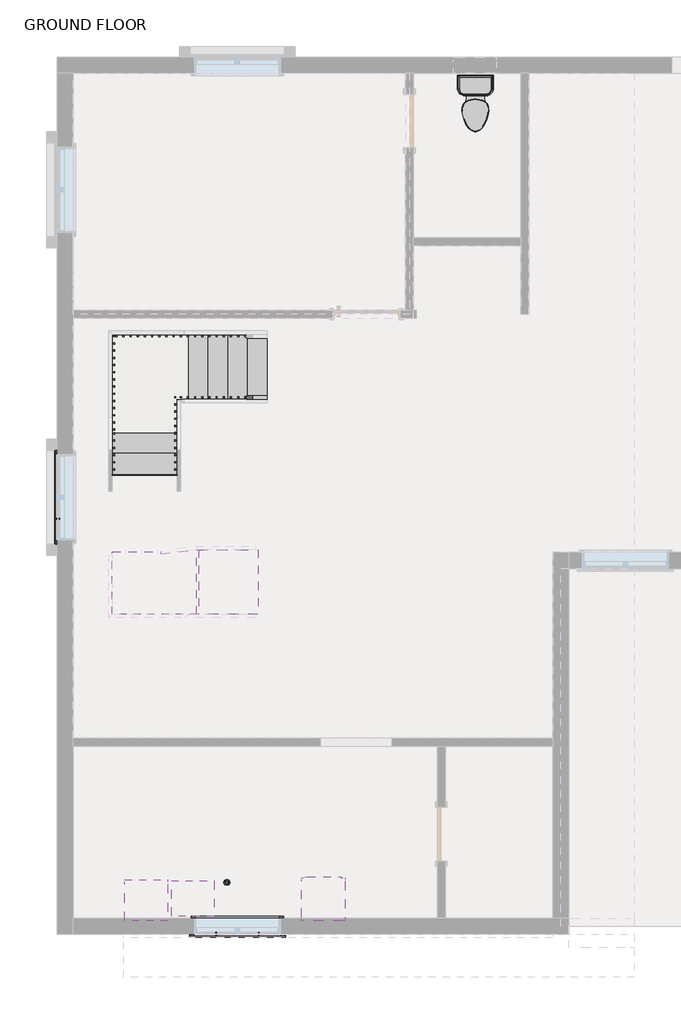
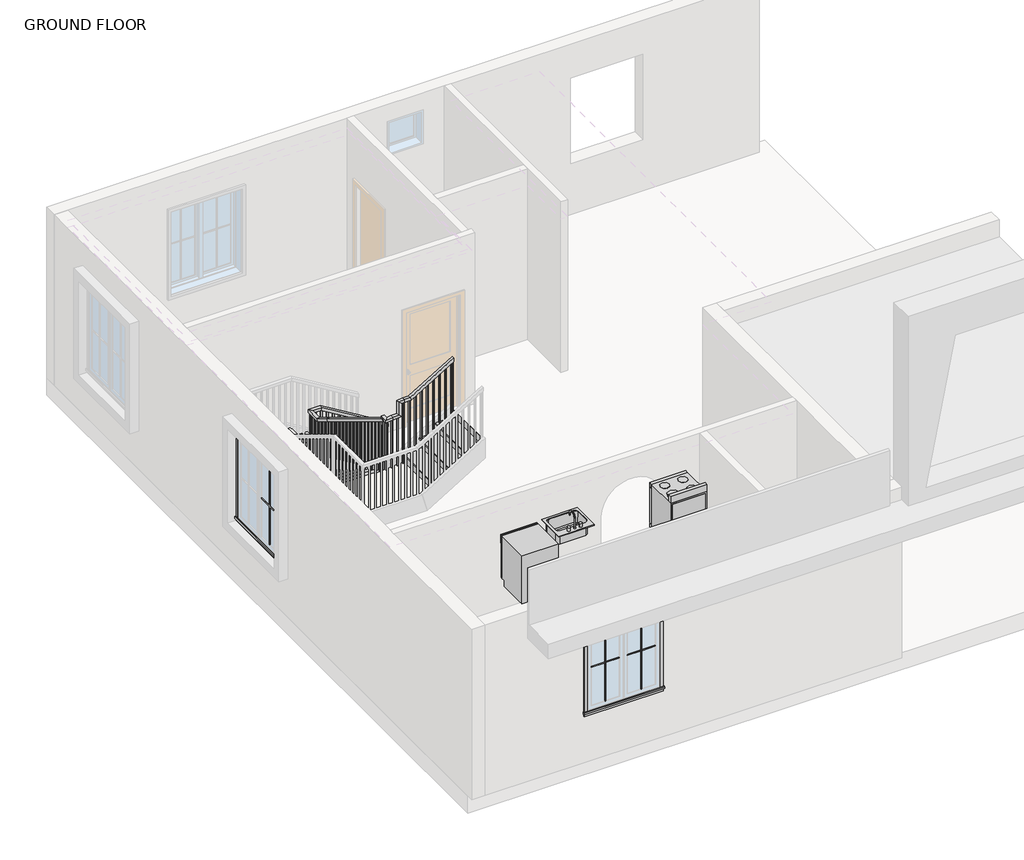
# One storey, part 3 of 4: 8 proxies, 3 flow terminals, 3 stair flights, 2 slabs, 1 railing.
"""IFC4 building model written with IfcOpenShell, lengths in millimetres."""

from ifc_helpers import new_model, si_unit, frame, origin, place, context, project, spatial, polyline, outline, extrude, faceted_brep, transform, mapped, element, save
from components import dishwasher_m_610_x_610_x_860mm_59039f12, muntin_pattern_2x2_muntin_pattern_2x2_6dad3731, muntin_pattern_2x2_muntin_pattern_2x2_a30a3345, range_m_610_x_610mm_7142e668, trim_window_exterior_flat_with_sill_92b9b949, trim_window_interior_flat_picture_frame_3bb882cf, flow_terminal_64mm_drain_64mm_drain_371441a0, m_sink_kitchen_single_760_x_535mm_2_7dd6f654, toilet_domestic_3d_toilet_domestic_3d_ba6479b0, toilet_domestic_3d_toilet_domestic_3d_30431060, non_monolithic_landing_bb2b3a88, non_monolithic_landing_7f41dad4, stair_flight_b4bfd778, stair_flight_23f0772b, stair_flight_a2e4d9b1

model = new_model("IFC4")

# Units and contexts
model_context = context("Model", 3, world=origin())
ifc_project = project(units=[si_unit("LENGTHUNIT", "METRE", prefix="MILLI")], contexts=[model_context])

# Site, building, storey
site = spatial("IfcSite", under=ifc_project)
building = spatial("IfcBuilding", under=site)
storey = spatial("IfcBuildingStorey", under=building, Name="GROUND FLOOR", Elevation=304.8)

# Proxies
placement = place(None, origin())
dishwasher_m_610_x_610_x_860mm_shape = dishwasher_m_610_x_610_x_860mm_59039f12(model_context)
element("IfcBuildingElementProxy", 1, Name="Dishwasher (M) : 610 x 610 x 860mm", ObjectType="Dishwasher (M) : 610 x 610 x 860mm", at=placement, inside=storey, context=model_context, shape_type="MappedRepresentation", body=[
    mapped(dishwasher_m_610_x_610_x_860mm_shape, transform((-11169.8760692, -6687.8348469, 3352.8), x_axis=(1.0, 0.0, 0.0), y_axis=(0.0, 1.0, 0.0), z_axis=(0.0, 0.0, 1.0))),
])
muntin_pattern_2x2_muntin_pattern_2x2_shape = muntin_pattern_2x2_muntin_pattern_2x2_6dad3731(model_context)
element("IfcBuildingElementProxy", 2, Name="Muntin Pattern_2x2 : Muntin Pattern_2x2", ObjectType="Muntin Pattern_2x2 : Muntin Pattern_2x2", at=placement, inside=storey, context=model_context, shape_type="MappedRepresentation", body=[
    mapped(muntin_pattern_2x2_muntin_pattern_2x2_shape, transform((-9193.7461008, -7440.4594117, 1289.05), x_axis=(-1.0, 0.0, 0.0), y_axis=(0.0, -1.0, 0.0), z_axis=(0.0, 0.0, 1.0))),
])
element("IfcBuildingElementProxy", 3, Name="Muntin Pattern_2x2 : Muntin Pattern_2x2", ObjectType="Muntin Pattern_2x2 : Muntin Pattern_2x2", at=placement, inside=storey, context=model_context, shape_type="MappedRepresentation", body=[
    mapped(muntin_pattern_2x2_muntin_pattern_2x2_shape, transform((-12040.1336008, -1561.9469117, 1289.05), x_axis=(0.0, 1.0, 0.0), y_axis=(-1.0, 0.0, 0.0), z_axis=(0.0, 0.0, 1.0))),
])
muntin_pattern_2x2_muntin_pattern_2x2_2_shape = muntin_pattern_2x2_muntin_pattern_2x2_a30a3345(model_context)
element("IfcBuildingElementProxy", 4, Name="Muntin Pattern_2x2 : Muntin Pattern_2x2", ObjectType="Muntin Pattern_2x2 : Muntin Pattern_2x2", at=placement, inside=storey, context=model_context, shape_type="MappedRepresentation", body=[
    mapped(muntin_pattern_2x2_muntin_pattern_2x2_2_shape, transform((-9800.1711008, -7440.4594117, 1289.05), x_axis=(1.0, 0.0, 0.0), y_axis=(0.0, 1.0, 0.0), z_axis=(0.0, 0.0, 1.0))),
])
range_m_610_x_610mm_shape = range_m_610_x_610mm_7142e668(model_context)
element("IfcBuildingElementProxy", 5, Name="Range (M) : 610 x 610mm", ObjectType="Range (M) : 610 x 610mm", at=placement, inside=storey, context=model_context, shape_type="MappedRepresentation", body=[
    mapped(range_m_610_x_610mm_shape, transform((-8584.7586008, -6649.4844117, 3352.8), x_axis=(1.0, 0.0, 0.0), y_axis=(0.0, 1.0, 0.0), z_axis=(0.0, 0.0, 1.0))),
])
trim_window_exterior_flat_with_sill_shape = trim_window_exterior_flat_with_sill_92b9b949(model_context)
element("IfcBuildingElementProxy", 6, Name="Trim-Window-Exterior-Flat : with Sill", ObjectType="Trim-Window-Exterior-Flat : with Sill", at=placement, inside=storey, context=model_context, shape_type="MappedRepresentation", body=[
    mapped(trim_window_exterior_flat_with_sill_shape, transform((-9496.9586008, -7449.9844117, 2743.2), x_axis=(1.0, 0.0, 0.0), y_axis=(0.0, 0.0, 1.0), z_axis=(0.0, -1.0, 0.0))),
])
element("IfcBuildingElementProxy", 7, Name="Trim-Window-Exterior-Flat : with Sill", ObjectType="Trim-Window-Exterior-Flat : with Sill", at=placement, inside=storey, context=model_context, shape_type="MappedRepresentation", body=[
    mapped(trim_window_exterior_flat_with_sill_shape, transform((-12049.6586008, -1258.7344117, 2743.2), x_axis=(0.0, -1.0, 0.0), y_axis=(0.0, 0.0, 1.0), z_axis=(-1.0, 0.0, 0.0))),
])
trim_window_interior_flat_picture_frame_shape = trim_window_interior_flat_picture_frame_3bb882cf(model_context)
element("IfcBuildingElementProxy", 8, Name="Trim-Window-Interior-Flat : Picture Frame", ObjectType="Trim-Window-Interior-Flat : Picture Frame", at=placement, inside=storey, context=model_context, shape_type="MappedRepresentation", body=[
    mapped(trim_window_interior_flat_picture_frame_shape, transform((-9496.9586008, -7221.3844117, 2743.2), x_axis=(-1.0, 0.0, 0.0), y_axis=(0.0, 0.0, 1.0), z_axis=(0.0, 1.0, 0.0))),
])

# Flow terminals
flow_terminal_64mm_drain_64mm_drain_shape = flow_terminal_64mm_drain_64mm_drain_371441a0(model_context)
element("IfcFlowTerminal", 9, ObjectType="64mm Drain : 64mm Drain", at=placement, inside=storey, context=model_context, shape_type="MappedRepresentation", body=[
    mapped(flow_terminal_64mm_drain_64mm_drain_shape, transform((-9497.2638536, -6711.8269352, 1092.2555314), x_axis=(1.0, 0.0, 0.0), y_axis=(0.0, 1.0, 0.0), z_axis=(0.0, 0.0, 1.0))),
])
m_sink_kitchen_single_760_x_535mm_2_shape = m_sink_kitchen_single_760_x_535mm_2_7dd6f654(model_context)
element("IfcFlowTerminal", 10, ObjectType="M_Sink Kitchen-Single : 760 x 535mm 2", at=placement, inside=storey, context=model_context, shape_type="MappedRepresentation", body=[
    mapped(m_sink_kitchen_single_760_x_535mm_2_shape, transform((-10114.0693602, -6939.4390106, 3352.8), x_axis=(-1.0, 0.0, 0.0), y_axis=(0.0, -1.0, 0.0), z_axis=(0.0, 0.0, 1.0))),
])
toilet_domestic_3d_toilet_domestic_3d_shape = toilet_domestic_3d_toilet_domestic_3d_ba6479b0(model_context)
toilet_domestic_3d_toilet_domestic_3d_2_shape = toilet_domestic_3d_toilet_domestic_3d_30431060(model_context)
element("IfcFlowTerminal", 11, ObjectType="Toilet-Domestic-3D : Toilet-Domestic-3D", at=placement, inside=storey, context=model_context, shape_type="MappedRepresentation", body=[
    mapped(toilet_domestic_3d_toilet_domestic_3d_shape, transform((-6125.1086008, 4221.3155883, 304.8), x_axis=(1.0, 0.0, 0.0), y_axis=(0.0, 1.0, 0.0), z_axis=(0.0, 0.0, 1.0))),
    mapped(toilet_domestic_3d_toilet_domestic_3d_2_shape, transform((-6125.1086008, 4221.3155883, 304.8), x_axis=(1.0, 0.0, 0.0), y_axis=(0.0, 1.0, 0.0), z_axis=(0.0, 0.0, 1.0))),
])

# Railing
element("IfcRailing", 12, ObjectType="Handrail - Rectangular", at=placement, inside=storey, context=model_context, shape_type="SolidModel", body=[
    faceted_brep([(-9079.7156858, 130.7115003, 1388.5333333), (-9079.7156858, 130.7115003, 1329.1318731), (-9079.7156858, 181.5115003, 1329.1318731), (-9079.7156858, 181.5115003, 1388.5333333), (-10197.3156858, 130.7115003, 2065.8666667), (-10211.5080953, 130.7115003, 2015.0666667), (-10211.5080953, 181.5115003, 2015.0666667), (-10197.3156858, 181.5115003, 2065.8666667), (-10353.7522729, 130.7115003, 2065.8666667), (-10353.7522729, 130.7115003, 2015.0666667), (-10404.5522729, 181.5115003, 2015.0666667), (-10404.5522729, 181.5115003, 2065.8666667), (-10353.7522729, -76.9993654, 2065.8666667), (-10353.7522729, -91.1917748, 2015.0666667), (-10404.5522729, -91.1917748, 2015.0666667), (-10404.5522729, -76.9993654, 2065.8666667), (-10353.7522729, -356.3993654, 2235.2), (-10353.7522729, -382.7290926, 2191.7559502), (-10404.5522729, -382.7290926, 2191.7559502), (-10404.5522729, -356.3993654, 2235.2), (-10353.7522729, -1959.5850154, 3206.8276667), (-10353.7522729, -2010.3850154, 3178.2140852), (-10404.5522729, -2010.3850154, 3178.2140852), (-10404.5522729, -1959.5850154, 3206.8276667), (-10353.7522729, -1959.5850154, 3251.2), (-10353.7522729, -2010.3850154, 3200.4), (-10404.5522729, -2010.3850154, 3200.4), (-10404.5522729, -1959.5850154, 3251.2), (-10353.7522729, -2032.7993654, 3251.2), (-10353.7522729, -2032.7993654, 3200.4), (-10404.5522729, -2089.5706654, 3200.4), (-10404.5522729, -2089.5706654, 3251.2), (-10280.987739, -2024.6960544, 3251.2), (-10280.987739, -2024.6960544, 3200.4), (-10275.3652319, -2075.1839481, 3200.4), (-10275.3652319, -2075.1839481, 3251.2), (-10176.7293559, -2013.085479, 3251.2), (-10126.2414621, -2007.4629719, 3200.4), (-10120.6189551, -2057.9508656, 3200.4), (-10171.1068488, -2063.5733727, 3251.2), (-10176.7293559, -2013.085479, 3482.9636109), (-10126.2414621, -2007.4629719, 3432.1636109), (-10120.6189551, -2057.9508656, 3432.1636109), (-10171.1068488, -2063.5733727, 3482.9636109), (-10074.3522729, -2001.6844117, 3482.9636109), (-10074.3522729, -2001.6844117, 3432.1636109), (-10071.5323568, -2052.4844117, 3432.1636109), (-10071.5323568, -2052.4844117, 3482.9636109), (-9971.3423149, -2001.6844117, 3482.9636109), (-9957.1499054, -2001.6844117, 3432.1636109), (-9957.1499054, -2052.4844117, 3432.1636109), (-9971.3423149, -2052.4844117, 3482.9636109), (-9236.1522729, -2001.6844117, 3928.5333333), (-9236.1522729, -2052.4844117, 3928.5333333), (-9236.1522729, -2052.4844117, 3869.1318731), (-9236.1522729, -2001.6844117, 3869.1318731)], [[[0, 1, 2, 3]], [[1, 0, 4, 5]], [[2, 1, 5, 6]], [[3, 2, 6, 7]], [[0, 3, 7, 4]], [[5, 4, 8, 9]], [[6, 5, 9, 10]], [[7, 6, 10, 11]], [[4, 7, 11, 8]], [[9, 8, 12, 13]], [[10, 9, 13, 14]], [[11, 10, 14, 15]], [[8, 11, 15, 12]], [[13, 12, 16, 17]], [[14, 13, 17, 18]], [[15, 14, 18, 19]], [[12, 15, 19, 16]], [[17, 16, 20, 21]], [[18, 17, 21, 22]], [[19, 18, 22, 23]], [[16, 19, 23, 20]], [[21, 20, 24, 25]], [[22, 21, 25, 26]], [[23, 22, 26, 27]], [[20, 23, 27, 24]], [[25, 24, 28, 29]], [[26, 25, 29, 30]], [[27, 26, 30, 31]], [[24, 27, 31, 28]], [[29, 28, 32, 33]], [[30, 29, 33, 34]], [[31, 30, 34, 35]], [[28, 31, 35, 32]], [[33, 32, 36, 37]], [[34, 33, 37, 38]], [[35, 34, 38, 39]], [[32, 35, 39, 36]], [[37, 36, 40, 41]], [[38, 37, 41, 42]], [[39, 38, 42, 43]], [[36, 39, 43, 40]], [[41, 40, 44, 45]], [[42, 41, 45, 46]], [[43, 42, 46, 47]], [[40, 43, 47, 44]], [[45, 44, 48, 49]], [[46, 45, 49, 50]], [[47, 46, 50, 51]], [[44, 47, 51, 48]], [[52, 53, 54, 55]], [[49, 48, 52, 55]], [[50, 49, 55, 54]], [[51, 50, 54, 53]], [[48, 51, 53, 52]]]),
    extrude(outline(polyline([(3848.8197264, -9269.6673149), (2844.8, -9269.6673149), (2844.8, -9250.6173149), (3860.365181, -9250.6173149), (3848.8197264, -9269.6673149)])), frame((0.0, -2036.6094117, 0.0), z_axis=(0.0, 1.0, 0.0), x_axis=(0.0, 0.0, 1.0)), (0.0, 0.0, 1.0), 19.05),
    extrude(outline(polyline([(3787.2714589, -9371.2673149), (2844.8, -9371.2673149), (2844.8, -9352.2173149), (3798.9612316, -9352.2173149), (3787.2714589, -9371.2673149)])), frame((0.0, -2036.6094117, 0.0), z_axis=(0.0, 1.0, 0.0), x_axis=(0.0, 0.0, 1.0)), (0.0, 0.0, 1.0), 19.05),
    extrude(outline(polyline([(3725.6682113, -9472.8673149), (2844.8, -9472.8673149), (2844.8, -9453.8173149), (3737.2136658, -9453.8173149), (3725.6682113, -9472.8673149)])), frame((0.0, -2036.6094117, 0.0), z_axis=(0.0, 1.0, 0.0), x_axis=(0.0, 0.0, 1.0)), (0.0, 0.0, 1.0), 19.05),
    extrude(outline(polyline([(3664.0924537, -9574.4673149), (2675.4666667, -9574.4673149), (2675.4666667, -9555.4173149), (3675.6379083, -9555.4173149), (3664.0924537, -9574.4673149)])), frame((0.0, -2036.6094117, 0.0), z_axis=(0.0, 1.0, 0.0), x_axis=(0.0, 0.0, 1.0)), (0.0, 0.0, 1.0), 19.05),
    extrude(outline(polyline([(3602.3517619, -9676.0673149), (2675.4666667, -9676.0673149), (2675.4666667, -9657.0173149), (3614.0415346, -9657.0173149), (3602.3517619, -9676.0673149)])), frame((0.0, -2036.6094117, 0.0), z_axis=(0.0, 1.0, 0.0), x_axis=(0.0, 0.0, 1.0)), (0.0, 0.0, 1.0), 19.05),
    extrude(outline(polyline([(3540.8715089, -9777.6673149), (2675.4666667, -9777.6673149), (2675.4666667, -9758.6173149), (3552.5612816, -9758.6173149), (3540.8715089, -9777.6673149)])), frame((0.0, -2036.6094117, 0.0), z_axis=(0.0, 1.0, 0.0), x_axis=(0.0, 0.0, 1.0)), (0.0, 0.0, 1.0), 19.05),
    extrude(outline(polyline([(3479.365181, -9879.2673149), (2506.1333333, -9879.2673149), (2506.1333333, -9860.2173149), (3490.9106355, -9860.2173149), (3479.365181, -9879.2673149)])), frame((0.0, -2036.6094117, 0.0), z_axis=(0.0, 1.0, 0.0), x_axis=(0.0, 0.0, 1.0)), (0.0, 0.0, 1.0), 19.05),
    extrude(outline(polyline([(3417.7894234, -9980.8673149), (2506.1333333, -9980.8673149), (2506.1333333, -9961.8173149), (3429.334878, -9961.8173149), (3417.7894234, -9980.8673149)])), frame((0.0, -2036.6094117, 0.0), z_axis=(0.0, 1.0, 0.0), x_axis=(0.0, 0.0, 1.0)), (0.0, 0.0, 1.0), 19.05),
    extrude(outline(polyline([(-10086.7456106, -2019.0377129), (-10067.8126505, -2016.9292728), (-10065.7042103, -2035.8622329), (-10084.6371705, -2037.9706731), (-10086.7456106, -2019.0377129)])), frame((0.0, 0.0, 2336.8), z_axis=(0.0, 0.0, 1.0), x_axis=(1.0, 0.0, 0.0)), (0.0, 0.0, 1.0), 1095.3636109),
    extrude(outline(polyline([(-10187.7213981, -2030.2827271), (-10168.7884379, -2028.1742869), (-10166.6799978, -2047.1072471), (-10185.6129579, -2049.2156872), (-10187.7213981, -2030.2827271)])), frame((0.0, 0.0, 2336.8), z_axis=(0.0, 0.0, 1.0), x_axis=(1.0, 0.0, 0.0)), (0.0, 0.0, 1.0), 863.6),
    extrude(outline(polyline([(-10288.6971856, -2041.5277412), (-10269.7642254, -2039.4193011), (-10267.6557853, -2058.3522612), (-10286.5887454, -2060.4607014), (-10288.6971856, -2041.5277412)])), frame((0.0, 0.0, 2336.8), z_axis=(0.0, 0.0, 1.0), x_axis=(1.0, 0.0, 0.0)), (0.0, 0.0, 1.0), 863.6),
    extrude(outline(polyline([(-10369.6272729, -1972.4743654), (-10369.6272729, -1991.5243654), (-10388.6772729, -1991.5243654), (-10388.6772729, -1972.4743654), (-10369.6272729, -1972.4743654)])), frame((0.0, 0.0, 2167.4666667), z_axis=(0.0, 0.0, 1.0), x_axis=(1.0, 0.0, 0.0)), (0.0, 0.0, 1.0), 1032.9333333),
    extrude(outline(polyline([(-1870.8743654, 3093.6621761), (-1870.8743654, 2167.4666667), (-1889.9243654, 2167.4666667), (-1889.9243654, 3105.2076307), (-1870.8743654, 3093.6621761)])), frame((-10388.6772729, 0.0, 0.0), z_axis=(1.0, 0.0, 0.0), x_axis=(0.0, 1.0, 0.0)), (0.0, 0.0, 1.0), 19.05),
    extrude(outline(polyline([(-1769.2743654, 3032.0063073), (-1769.2743654, 2167.4666667), (-1788.3243654, 2167.4666667), (-1788.3243654, 3043.6960801), (-1769.2743654, 3032.0063073)])), frame((-10388.6772729, 0.0, 0.0), z_axis=(1.0, 0.0, 0.0), x_axis=(0.0, 1.0, 0.0)), (0.0, 0.0, 1.0), 19.05),
    extrude(outline(polyline([(-1667.6743654, 2970.510661), (-1667.6743654, 1998.1333333), (-1686.7243654, 1998.1333333), (-1686.7243654, 2982.0561155), (-1667.6743654, 2970.510661)])), frame((-10388.6772729, 0.0, 0.0), z_axis=(1.0, 0.0, 0.0), x_axis=(0.0, 1.0, 0.0)), (0.0, 0.0, 1.0), 19.05),
    extrude(outline(polyline([(-1566.0743654, 2908.9349034), (-1566.0743654, 1998.1333333), (-1585.1243654, 1998.1333333), (-1585.1243654, 2920.4803579), (-1566.0743654, 2908.9349034)])), frame((-10388.6772729, 0.0, 0.0), z_axis=(1.0, 0.0, 0.0), x_axis=(0.0, 1.0, 0.0)), (0.0, 0.0, 1.0), 19.05),
    extrude(outline(polyline([(-1464.4743654, 2847.3591458), (-1464.4743654, 1998.1333333), (-1483.5243654, 1998.1333333), (-1483.5243654, 2858.9046004), (-1464.4743654, 2847.3591458)])), frame((-10388.6772729, 0.0, 0.0), z_axis=(1.0, 0.0, 0.0), x_axis=(0.0, 1.0, 0.0)), (0.0, 0.0, 1.0), 19.05),
    extrude(outline(polyline([(-1362.8743654, 2785.7833882), (-1362.8743654, 1828.8), (-1381.9243654, 1828.8), (-1381.9243654, 2797.3288428), (-1362.8743654, 2785.7833882)])), frame((-10388.6772729, 0.0, 0.0), z_axis=(1.0, 0.0, 0.0), x_axis=(0.0, 1.0, 0.0)), (0.0, 0.0, 1.0), 19.05),
    extrude(outline(polyline([(-1261.2743654, 2724.2076307), (-1261.2743654, 1828.8), (-1280.3243654, 1828.8), (-1280.3243654, 2735.7530852), (-1261.2743654, 2724.2076307)])), frame((-10388.6772729, 0.0, 0.0), z_axis=(1.0, 0.0, 0.0), x_axis=(0.0, 1.0, 0.0)), (0.0, 0.0, 1.0), 19.05),
    extrude(outline(polyline([(-1159.6743654, 2662.6318731), (-1159.6743654, 1659.4666667), (-1178.7243654, 1659.4666667), (-1178.7243654, 2674.1773276), (-1159.6743654, 2662.6318731)])), frame((-10388.6772729, 0.0, 0.0), z_axis=(1.0, 0.0, 0.0), x_axis=(0.0, 1.0, 0.0)), (0.0, 0.0, 1.0), 19.05),
    extrude(outline(polyline([(-1058.0743654, 2601.0561155), (-1058.0743654, 1659.4666667), (-1077.1243654, 1659.4666667), (-1077.1243654, 2612.60157), (-1058.0743654, 2601.0561155)])), frame((-10388.6772729, 0.0, 0.0), z_axis=(1.0, 0.0, 0.0), x_axis=(0.0, 1.0, 0.0)), (0.0, 0.0, 1.0), 19.05),
    extrude(outline(polyline([(-956.4743654, 2539.4803579), (-956.4743654, 1659.4666667), (-975.5243654, 1659.4666667), (-975.5243654, 2551.0258125), (-956.4743654, 2539.4803579)])), frame((-10388.6772729, 0.0, 0.0), z_axis=(1.0, 0.0, 0.0), x_axis=(0.0, 1.0, 0.0)), (0.0, 0.0, 1.0), 19.05),
    extrude(outline(polyline([(-854.8743654, 2477.9046004), (-854.8743654, 1490.1333333), (-873.9243654, 1490.1333333), (-873.9243654, 2489.4500549), (-854.8743654, 2477.9046004)])), frame((-10388.6772729, 0.0, 0.0), z_axis=(1.0, 0.0, 0.0), x_axis=(0.0, 1.0, 0.0)), (0.0, 0.0, 1.0), 19.05),
    extrude(outline(polyline([(-753.2743654, 2416.3288428), (-753.2743654, 1490.1333333), (-772.3243654, 1490.1333333), (-772.3243654, 2427.8742973), (-753.2743654, 2416.3288428)])), frame((-10388.6772729, 0.0, 0.0), z_axis=(1.0, 0.0, 0.0), x_axis=(0.0, 1.0, 0.0)), (0.0, 0.0, 1.0), 19.05),
    extrude(outline(polyline([(-651.6743654, 2354.672974), (-651.6743654, 1490.1333333), (-670.7243654, 1490.1333333), (-670.7243654, 2366.3627467), (-651.6743654, 2354.672974)])), frame((-10388.6772729, 0.0, 0.0), z_axis=(1.0, 0.0, 0.0), x_axis=(0.0, 1.0, 0.0)), (0.0, 0.0, 1.0), 19.05),
    extrude(outline(polyline([(-550.0743654, 2293.1773276), (-550.0743654, 1320.8), (-569.1243654, 1320.8), (-569.1243654, 2304.7227822), (-550.0743654, 2293.1773276)])), frame((-10388.6772729, 0.0, 0.0), z_axis=(1.0, 0.0, 0.0), x_axis=(0.0, 1.0, 0.0)), (0.0, 0.0, 1.0), 19.05),
    extrude(outline(polyline([(-448.4743654, 2231.60157), (-448.4743654, 1320.8), (-467.5243654, 1320.8), (-467.5243654, 2243.1470246), (-448.4743654, 2231.60157)])), frame((-10388.6772729, 0.0, 0.0), z_axis=(1.0, 0.0, 0.0), x_axis=(0.0, 1.0, 0.0)), (0.0, 0.0, 1.0), 19.05),
    extrude(outline(polyline([(-342.3634997, 2167.2919545), (-342.3634997, 1151.4666667), (-361.4134997, 1151.4666667), (-361.4134997, 2178.837409), (-342.3634997, 2167.2919545)])), frame((-10388.6772729, 0.0, 0.0), z_axis=(1.0, 0.0, 0.0), x_axis=(0.0, 1.0, 0.0)), (0.0, 0.0, 1.0), 19.05),
    extrude(outline(polyline([(-240.7634997, 2105.7161969), (-240.7634997, 1151.4666667), (-259.8134997, 1151.4666667), (-259.8134997, 2117.2616515), (-240.7634997, 2105.7161969)])), frame((-10388.6772729, 0.0, 0.0), z_axis=(1.0, 0.0, 0.0), x_axis=(0.0, 1.0, 0.0)), (0.0, 0.0, 1.0), 19.05),
    extrude(outline(polyline([(-139.1634997, 2044.1404393), (-139.1634997, 1151.4666667), (-158.2134997, 1151.4666667), (-158.2134997, 2055.6858939), (-139.1634997, 2044.1404393)])), frame((-10388.6772729, 0.0, 0.0), z_axis=(1.0, 0.0, 0.0), x_axis=(0.0, 1.0, 0.0)), (0.0, 0.0, 1.0), 19.05),
    extrude(outline(polyline([(-10369.6272729, -37.5634997), (-10369.6272729, -56.6134997), (-10388.6772729, -56.6134997), (-10388.6772729, -37.5634997), (-10369.6272729, -37.5634997)])), frame((0.0, 0.0, 1151.4666667), z_axis=(0.0, 0.0, 1.0), x_axis=(1.0, 0.0, 0.0)), (0.0, 0.0, 1.0), 863.6),
    extrude(outline(polyline([(-10369.6272729, 64.0365003), (-10369.6272729, 44.9865003), (-10388.6772729, 44.9865003), (-10388.6772729, 64.0365003), (-10369.6272729, 64.0365003)])), frame((0.0, 0.0, 1151.4666667), z_axis=(0.0, 0.0, 1.0), x_axis=(1.0, 0.0, 0.0)), (0.0, 0.0, 1.0), 863.6),
    extrude(outline(polyline([(-10289.3906858, 146.5865003), (-10308.4406858, 146.5865003), (-10308.4406858, 165.6365003), (-10289.3906858, 165.6365003), (-10289.3906858, 146.5865003)])), frame((0.0, 0.0, 1151.4666667), z_axis=(0.0, 0.0, 1.0), x_axis=(1.0, 0.0, 0.0)), (0.0, 0.0, 1.0), 863.6),
    extrude(outline(polyline([(1950.6621761, -10105.2406858), (982.1333333, -10105.2406858), (982.1333333, -10086.1906858), (1939.1167216, -10086.1906858), (1950.6621761, -10105.2406858)])), frame((0.0, 146.5865003, 0.0), z_axis=(0.0, 1.0, 0.0), x_axis=(0.0, 0.0, 1.0)), (0.0, 0.0, 1.0), 19.05),
    extrude(outline(polyline([(1889.0864185, -10003.6406858), (982.1333333, -10003.6406858), (982.1333333, -9984.5906858), (1877.540964, -9984.5906858), (1889.0864185, -10003.6406858)])), frame((0.0, 146.5865003, 0.0), z_axis=(0.0, 1.0, 0.0), x_axis=(0.0, 0.0, 1.0)), (0.0, 0.0, 1.0), 19.05),
    extrude(outline(polyline([(1827.510661, -9902.0406858), (812.8, -9902.0406858), (812.8, -9882.9906858), (1815.9652064, -9882.9906858), (1827.510661, -9902.0406858)])), frame((0.0, 146.5865003, 0.0), z_axis=(0.0, 1.0, 0.0), x_axis=(0.0, 0.0, 1.0)), (0.0, 0.0, 1.0), 19.05),
    extrude(outline(polyline([(1765.9349034, -9800.4406858), (812.8, -9800.4406858), (812.8, -9781.3906858), (1754.3894488, -9781.3906858), (1765.9349034, -9800.4406858)])), frame((0.0, 146.5865003, 0.0), z_axis=(0.0, 1.0, 0.0), x_axis=(0.0, 0.0, 1.0)), (0.0, 0.0, 1.0), 19.05),
    extrude(outline(polyline([(1704.3591458, -9698.8406858), (812.8, -9698.8406858), (812.8, -9679.7906858), (1692.8136913, -9679.7906858), (1704.3591458, -9698.8406858)])), frame((0.0, 146.5865003, 0.0), z_axis=(0.0, 1.0, 0.0), x_axis=(0.0, 0.0, 1.0)), (0.0, 0.0, 1.0), 19.05),
    extrude(outline(polyline([(1642.7833882, -9597.2406858), (643.4666667, -9597.2406858), (643.4666667, -9578.1906858), (1631.2379337, -9578.1906858), (1642.7833882, -9597.2406858)])), frame((0.0, 146.5865003, 0.0), z_axis=(0.0, 1.0, 0.0), x_axis=(0.0, 0.0, 1.0)), (0.0, 0.0, 1.0), 19.05),
    extrude(outline(polyline([(1581.2076307, -9495.6406858), (643.4666667, -9495.6406858), (643.4666667, -9476.5906858), (1569.6621761, -9476.5906858), (1581.2076307, -9495.6406858)])), frame((0.0, 146.5865003, 0.0), z_axis=(0.0, 1.0, 0.0), x_axis=(0.0, 0.0, 1.0)), (0.0, 0.0, 1.0), 19.05),
    extrude(outline(polyline([(1519.6960801, -9394.0406858), (643.4666667, -9394.0406858), (643.4666667, -9374.9906858), (1508.0063073, -9374.9906858), (1519.6960801, -9394.0406858)])), frame((0.0, 146.5865003, 0.0), z_axis=(0.0, 1.0, 0.0), x_axis=(0.0, 0.0, 1.0)), (0.0, 0.0, 1.0), 19.05),
    extrude(outline(polyline([(1458.0561155, -9292.4406858), (474.1333333, -9292.4406858), (474.1333333, -9273.3906858), (1446.510661, -9273.3906858), (1458.0561155, -9292.4406858)])), frame((0.0, 146.5865003, 0.0), z_axis=(0.0, 1.0, 0.0), x_axis=(0.0, 0.0, 1.0)), (0.0, 0.0, 1.0), 19.05),
    extrude(outline(polyline([(1396.4803579, -9190.8406858), (474.1333333, -9190.8406858), (474.1333333, -9171.7906858), (1384.9349034, -9171.7906858), (1396.4803579, -9190.8406858)])), frame((0.0, 146.5865003, 0.0), z_axis=(0.0, 1.0, 0.0), x_axis=(0.0, 0.0, 1.0)), (0.0, 0.0, 1.0), 19.05),
    extrude(outline(polyline([(-10083.463015, -2018.6721517), (-10064.5300549, -2016.5637115), (-10062.4216147, -2035.4966717), (-10081.3545749, -2037.6051118), (-10083.463015, -2018.6721517)])), frame((0.0, 0.0, 2336.8), z_axis=(0.0, 0.0, 1.0), x_axis=(1.0, 0.0, 0.0)), (0.0, 0.0, 1.0), 1095.3636109),
    extrude(outline(polyline([(-10369.6272729, -2051.6600154), (-10369.6272729, -2070.7100154), (-10388.6772729, -2070.7100154), (-10388.6772729, -2051.6600154), (-10369.6272729, -2051.6600154)])), frame((0.0, 0.0, 2336.8), z_axis=(0.0, 0.0, 1.0), x_axis=(1.0, 0.0, 0.0)), (0.0, 0.0, 1.0), 863.6),
    extrude(outline(polyline([(-346.8743654, 2170.0258125), (-346.8743654, 1151.4666667), (-365.9243654, 1151.4666667), (-365.9243654, 2181.571267), (-346.8743654, 2170.0258125)])), frame((-10388.6772729, 0.0, 0.0), z_axis=(1.0, 0.0, 0.0), x_axis=(0.0, 1.0, 0.0)), (0.0, 0.0, 1.0), 19.05),
    extrude(outline(polyline([(-10369.6272729, 146.5865003), (-10388.6772729, 146.5865003), (-10388.6772729, 165.6365003), (-10369.6272729, 165.6365003), (-10369.6272729, 146.5865003)])), frame((0.0, 0.0, 1151.4666667), z_axis=(0.0, 0.0, 1.0), x_axis=(1.0, 0.0, 0.0)), (0.0, 0.0, 1.0), 863.6),
    extrude(outline(polyline([(2012.2379337, -10206.8406858), (1151.4666667, -10206.8406858), (1151.4666667, -10187.7906858), (2000.6924791, -10187.7906858), (2012.2379337, -10206.8406858)])), frame((0.0, 146.5865003, 0.0), z_axis=(0.0, 1.0, 0.0), x_axis=(0.0, 0.0, 1.0)), (0.0, 0.0, 1.0), 19.05),
    extrude(outline(polyline([(3857.5864185, -9255.2022729), (2844.8, -9255.2022729), (2844.8, -9236.1522729), (3869.1318731, -9236.1522729), (3857.5864185, -9255.2022729)])), frame((0.0, -2036.6094117, 0.0), z_axis=(0.0, 1.0, 0.0), x_axis=(0.0, 0.0, 1.0)), (0.0, 0.0, 1.0), 19.05),
    extrude(outline(polyline([(1340.6212695, -9098.7656858), (474.1333333, -9098.7656858), (474.1333333, -9079.7156858), (1328.9314967, -9079.7156858), (1340.6212695, -9098.7656858)])), frame((0.0, 146.5865003, 0.0), z_axis=(0.0, 1.0, 0.0), x_axis=(0.0, 0.0, 1.0)), (0.0, 0.0, 1.0), 19.05),
])

# Slabs
non_monolithic_landing_shape = non_monolithic_landing_bb2b3a88(model_context)
element("IfcSlab", 13, ObjectType="Non-Monolithic Landing", at=placement, inside=storey, context=model_context, shape_type="MappedRepresentation", body=[
    mapped(non_monolithic_landing_shape, transform((0.0, 0.0, 0.0), x_axis=(1.0, 0.0, 0.0), y_axis=(0.0, 1.0, 0.0), z_axis=(0.0, 0.0, 1.0))),
])
non_monolithic_landing_2_shape = non_monolithic_landing_7f41dad4(model_context)
element("IfcSlab", 14, ObjectType="Non-Monolithic Landing", at=placement, inside=storey, context=model_context, shape_type="MappedRepresentation", body=[
    mapped(non_monolithic_landing_2_shape, transform((0.0, 0.0, 0.0), x_axis=(1.0, 0.0, 0.0), y_axis=(0.0, 1.0, 0.0), z_axis=(0.0, 0.0, 1.0))),
])

# Stair flights
stair_flight_shape = stair_flight_b4bfd778(model_context)
element("IfcStairFlight", 15, ObjectType="2\" Tread 1\" Nosing 1/4\" Riser", at=placement, inside=storey, context=model_context, shape_type="MappedRepresentation", body=[
    mapped(stair_flight_shape, transform((0.0, 0.0, 0.0), x_axis=(1.0, 0.0, 0.0), y_axis=(0.0, 1.0, 0.0), z_axis=(0.0, 0.0, 1.0))),
])
stair_flight_2_shape = stair_flight_23f0772b(model_context)
element("IfcStairFlight", 16, ObjectType="2\" Tread 1\" Nosing 1/4\" Riser", at=placement, inside=storey, context=model_context, shape_type="MappedRepresentation", body=[
    mapped(stair_flight_2_shape, transform((0.0, 0.0, 0.0), x_axis=(1.0, 0.0, 0.0), y_axis=(0.0, 1.0, 0.0), z_axis=(0.0, 0.0, 1.0))),
])
stair_flight_3_shape = stair_flight_a2e4d9b1(model_context)
element("IfcStairFlight", 17, ObjectType="2\" Tread 1\" Nosing 1/4\" Riser", at=placement, inside=storey, context=model_context, shape_type="MappedRepresentation", body=[
    mapped(stair_flight_3_shape, transform((0.0, 0.0, 0.0), x_axis=(1.0, 0.0, 0.0), y_axis=(0.0, 1.0, 0.0), z_axis=(0.0, 0.0, 1.0))),
])

save(model, "model.ifc")

# Revit data of these elements
# Type "Dishwasher (M) : 610 x 610 x 860mm"
#   Label = "DW"
#   Depth = 2' - 0.01575"
#   Height = 2' - 9.85827"
#   Width = 2' - 0.01575"
#   Dishwasher Material = Metal - Paint Finish - Ivory,Glossy
#   Panel Face Material = Plastic - Black
#   Default Elevation = 0
# Type "Muntin Pattern_2x2 : Muntin Pattern_2x2"
#   Width [instance default] = 4' - 0"
#   Thickness = 0' - 0 1/2"
#   Height [instance default] = 4' - 0"
#   Distance = 0' - 0 3/4"
#   Interior Material [instance default] = none
#   Exterior Material [instance default] = none
#   Default Elevation = 0
# Type "Range (M) : 610 x 610mm"
#   Depth = 2' - 0.01575"
#   Width = 2' - 0.01575"
#   Burner Material = Metal - Chrome
#   Range Material = Metal - Painted Finish - Ivory,Matte
#   Default Elevation = 0
#   Assembly Code = ""
# Type "Trim-Window-Exterior-Flat : with Sill"
#   Trim Width = 0' - 2 1/4"
#   Trim Thickness_Picture Frame = 0' - 1 1/4"
#   Trim Thickness_with Sill = 0' - 0 3/4"
#   Sill Thickness = 0' - 1 1/4"
#   Opening Width [instance default] = 2' - 0"
#   Opening Height [instance default] = 3' - 0"
#   Default Elevation = 4' - 0"
#   Sill = yes
#   Picture Frame = no
#   Trim Material [instance default] = none
# Type "Trim-Window-Interior-Flat : Picture Frame"
#   Trim Thickness_Picture Frame = 0' - 1 1/4"
#   Trim Width = 0' - 2 1/4"
#   Trim Thickness_with Sill = 0' - 0 3/4"
#   Sill Thickness = 0' - 1 1/4"
#   Opening Width [instance default] = 2' - 0"
#   Opening Height [instance default] = 3' - 0"
#   Default Elevation = 4' - 0"
#   Sill = no
#   Picture Frame = yes
#   Trim Material [instance default] = none
# Type "64mm Drain : 64mm Drain"
#   Finish = none
#   Default Elevation = 0
#   Assembly Code = ""
# Type "M_Sink Kitchen-Single : 760 x 535mm 2"
#   Counter Height = 3' - 0.22047"
#   Depth = 1' - 7.68504"
#   Width = 1' - 11.62205"
#   Fixture Material = Metal - Steel, Polished
#   Sink Material = Metal - Steel, Polished
#   Default Elevation = 0
#   Assembly Code = ""
# Type "Toilet-Domestic-3D : Toilet-Domestic-3D"
#   Assembly Code = "D2010110"
#   Toilet - Bowl/Basin Material = Porcelain, Linen
#   Toilet - Seat Material = Laminate, Linen, Matte
#   Default Elevation = 0
# Type "Handrail - Rectangular"
#   Assembly Code = "C2010400"
#   built-in parameter 1008612 = 0.0416667 (stored number, unit not read)
#   built-in parameter 1008611 = 0.0416667 (stored number, unit not read)
#   built-in parameter 1008609 = 0.333333 (stored number, unit not read)
#   built-in parameter 1008604 = 0.166667 (stored number, unit not read)
#   built-in parameter 1008603 = 0.166667 (stored number, unit not read)
#   Railing Height = 3' - 0"
#   built-in parameter 1008630 = 2
#   built-in parameter 1008610 = 2
#   built-in parameter 1008618 = Baluster - Square : 3/4"
# Element 1 (IfcBuildingElementProxy, "Dishwasher (M) : 610 x 610 x 860mm")
#   Phase Created = New Construction
#   Materials on its faces: "Metal - Paint Finish - Ivory,Glossy", "Plastic - Black"
# Elements 2, 3, 4 (IfcBuildingElementProxy, "Muntin Pattern_2x2 : Muntin Pattern_2x2")
#   Width = 1' - 6 5/8"
#   Height = 4' - 6 1/2"
#   Interior Material = Wood - Stained
#   Exterior Material = BLACK MATERIAL
#   Phase Created = New Construction
#   Materials on its faces: "BLACK MATERIAL", "Wood - Stained"
# Element 5 (IfcBuildingElementProxy, "Range (M) : 610 x 610mm")
#   Phase Created = New Construction
#   Materials on its faces: "Metal - Painted Finish - Ivory,Matte", "Metal - Chrome", "Glass"
# Elements 6, 7 (IfcBuildingElementProxy, "Trim-Window-Exterior-Flat : with Sill")
#   Opening Width = 4' - 0"
#   Opening Height = 5' - 0"
#   Trim Material = BLACK MATERIAL
#   Phase Created = New Construction
#   Materials on its faces: "BLACK MATERIAL"
# Element 8 (IfcBuildingElementProxy, "Trim-Window-Interior-Flat : Picture Frame")
#   Opening Width = 4' - 0"
#   Opening Height = 5' - 0"
#   Trim Material = Wood - Stained
#   Phase Created = New Construction
#   Materials on its faces: "Wood - Stained"
# Element 9 (IfcFlowTerminal, "64mm Drain : 64mm Drain")
#   Mark = "1"
#   Phase Created = New Construction
#   Materials on its faces: "Polished Chrome"
# Element 10 (IfcFlowTerminal, "M_Sink Kitchen-Single : 760 x 535mm 2")
#   Mark = "5"
#   Phase Created = New Construction
#   Materials on its faces: "Metal - Steel, Polished"
# Element 11 (IfcFlowTerminal, "Toilet-Domestic-3D : Toilet-Domestic-3D")
#   Mark = "3"
#   Phase Created = New Construction
#   Materials on its faces: "Porcelain, Linen", "Laminate, Linen, Matte"
# Element 12 (IfcRailing, "Handrail - Rectangular")
#   Phase Created = New Construction
# Elements 13, 14 (IfcSlab, "Non-Monolithic Landing")
#   Phase Created = New Construction
# Elements 15, 16, 17 (IfcStairFlight, "2\" Tread 1\" Nosing 1/4\" Riser")
#   Phase Created = New Construction
# Materials
#   "Metal - Paint Finish - Ivory,Glossy": colour RGB 247 247 239, transparency 0
#   "Plastic - Black": colour RGB 0 0 0, transparency 0.7
#   "Metal - Chrome": colour RGB 17 17 17, transparency 0
#   "Metal - Painted Finish - Ivory,Matte": colour RGB 247 247 239, transparency 0
#   "Metal - Steel, Polished": class "Metal", colour RGB 192 192 192, transparency 0
#   "Porcelain, Linen": class "Ceramic", colour RGB 249 239 230, transparency 0, Description = "Porcelain, linen", Cost = 0
#   "Laminate, Linen, Matte": class "Plastic", colour RGB 249 239 230, transparency 0, Description = "Plastic Laminate - Linen, Matte", Cost = 0
#   "BLACK MATERIAL": class "Generic", colour RGB 120 120 120, transparency 0, Cost = 0
#   "Wood - Stained": class "Wood", colour RGB 224 178 126, transparency 0, Cost = 0
#   "Glass": class "Glass", colour RGB 0 128 192, transparency 0.75, Description = "Soda Lime Glass", Cost = 0
#   "Polished Chrome": colour RGB 247 247 247, transparency 0
